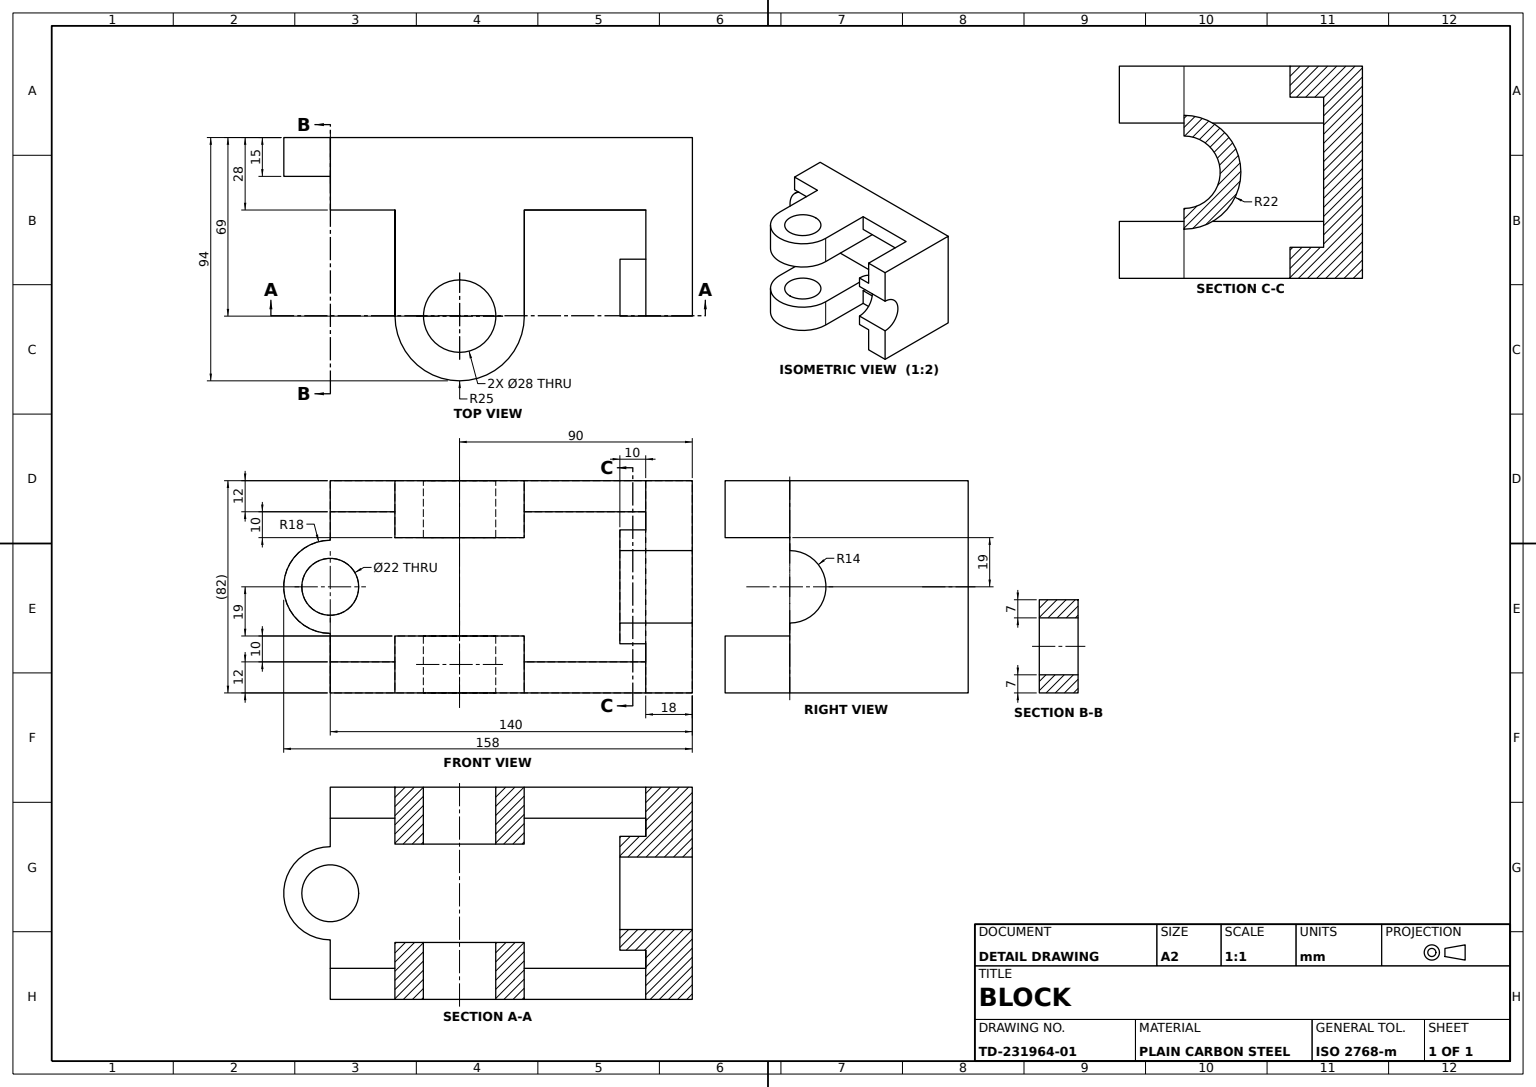
from build123d import *

# Parameters (mm, degrees)
BASE_PLATE_SKETCH_W         = 140
BASE_PLATE_SKETCH_H         = 82
BASE_PLATE_DEPTH            = 15
BACK_WALL_SKETCH_W          = 54
BACK_WALL_SKETCH_H          = 82
BACK_WALL_DEPTH             = 18
REAR_HALF_BOSS_DEPTH        = 10
REAR_HALF_ROUND_CUT_DEPTH   = 28
LOWER_LUG_DEPTH             = 22
SPACER_BLOCK_1_SKETCH_W     = 47
SPACER_BLOCK_1_SKETCH_H     = 13
SPACER_BLOCK_1_DEPTH        = 12
SPACER_BLOCK_2_SKETCH_W     = 25
SPACER_BLOCK_2_SKETCH_H     = 13
SPACER_BLOCK_2_DEPTH        = 12
SPACER_BLOCK_3_SKETCH_W     = 47
SPACER_BLOCK_3_SKETCH_H     = 13
SPACER_BLOCK_3_DEPTH        = 12
UPPER_START                 = -22
UPPER_LUG_DEPTH             = 22
SPACER_BLOCK_4_SKETCH_W     = 25
SPACER_BLOCK_4_SKETCH_H     = 13
SPACER_BLOCK_4_DEPTH        = 12
SIDE_HALF_BOSS_DEPTH        = 15
SIDE_BORE_SKETCH_R          = 11
SIDE_BORE_22_DEPTH          = 15
UPPER_PIN_HOLE_SKETCH_R     = 14
UPPER_LUG_PIN_HOLE_28_DEPTH = 22
LOWER_START                 = -22
LOWER_PIN_HOLE_SKETCH_R     = 14
LOWER_LUG_PIN_HOLE_28_DEPTH = 22


with BuildPart() as part:
    # Base Plate Sketch → Base Plate (new body)
    with BuildSketch(Plane.XY):
        with Locations((70, 41)):
            Rectangle(BASE_PLATE_SKETCH_W, BASE_PLATE_SKETCH_H)
    extrude(amount=BASE_PLATE_DEPTH)

    # Back Wall Sketch → Back Wall (add)
    with BuildSketch(Plane(origin=(140, 0, 0), x_dir=(0, 0, -1), z_dir=(1, 0, 0))):
        with Locations((-42, 41)):
            Rectangle(BACK_WALL_SKETCH_W, BACK_WALL_SKETCH_H)
    extrude(amount=-BACK_WALL_DEPTH)

    # Rear Half Boss Sketch → Rear Half Boss (add)
    with BuildSketch(Plane.ZY.offset(-122)):
        with BuildLine():
            Line((69, 63), (69, 19))
            ThreePointArc((69, 19), (47, 41), (69, 63))
        make_face()
    extrude(amount=REAR_HALF_BOSS_DEPTH)

    # Rear Half-Round Cut Sketch → Rear Half-Round Cut (cut)
    with BuildSketch(Plane.ZY.offset(-112)):
        with BuildLine():
            Line((69, 55), (69, 27))
            ThreePointArc((69, 27), (55, 41), (69, 55))
        make_face()
    extrude(amount=-REAR_HALF_ROUND_CUT_DEPTH, mode=Mode.SUBTRACT)

    # Lower Lug Sketch → Lower Lug (add)
    with BuildSketch(Plane.XZ):
        with BuildLine():
            Line((75, 69), (75, 15))
            Line((75, 15), (25, 15))
            Line((25, 15), (25, 69))
            ThreePointArc((25, 69), (50, 94), (75, 69))
        make_face()
    extrude(amount=-LOWER_LUG_DEPTH)

    # Spacer Block 1 Sketch → Spacer Block 1 (add)
    with BuildSketch(Plane.XZ):
        with Locations((98.5, 21.5)):
            Rectangle(SPACER_BLOCK_1_SKETCH_W, SPACER_BLOCK_1_SKETCH_H)
    extrude(amount=-SPACER_BLOCK_1_DEPTH)

    # Spacer Block 2 Sketch → Spacer Block 2 (add)
    with BuildSketch(Plane.XZ):
        with Locations((12.5, 21.5)):
            Rectangle(SPACER_BLOCK_2_SKETCH_W, SPACER_BLOCK_2_SKETCH_H)
    extrude(amount=-SPACER_BLOCK_2_DEPTH)

    # Spacer Block 3 Sketch → Spacer Block 3 (add)
    with BuildSketch(Plane(origin=(0, 82, 0), x_dir=(1, 0, 0), z_dir=(0, 1, 0))):
        with Locations((98.5, -21.5)):
            Rectangle(SPACER_BLOCK_3_SKETCH_W, SPACER_BLOCK_3_SKETCH_H)
    extrude(amount=-SPACER_BLOCK_3_DEPTH)

    # Upper Lug Sketch → Upper Lug (add)
    with BuildSketch(Plane(origin=(0, 82, 0), x_dir=(1, 0, 0), z_dir=(0, 1, 0)).offset(UPPER_START)):
        with BuildLine():
            Line((25, -15), (75, -15))
            Line((75, -15), (75, -69))
            ThreePointArc((75, -69), (50, -94), (25, -69))
            Line((25, -69), (25, -15))
        make_face()
    extrude(amount=UPPER_LUG_DEPTH)

    # Spacer Block 4 Sketch → Spacer Block 4 (add)
    with BuildSketch(Plane(origin=(0, 82, 0), x_dir=(1, 0, 0), z_dir=(0, 1, 0))):
        with Locations((12.5, -21.5)):
            Rectangle(SPACER_BLOCK_4_SKETCH_W, SPACER_BLOCK_4_SKETCH_H)
    extrude(amount=-SPACER_BLOCK_4_DEPTH)

    # Side Half Boss Sketch → Side Half Boss (add)
    with BuildSketch(Plane.XY.offset(15)):
        with BuildLine():
            Line((0, 59), (0, 23))
            ThreePointArc((0, 23), (-18, 41), (0, 59))
        make_face()
    extrude(amount=-SIDE_HALF_BOSS_DEPTH)

    # Side Bore Sketch → Side Bore Ø22 (cut)
    with BuildSketch(Plane.XY.offset(15)):
        with Locations((0, 41)):
            Circle(SIDE_BORE_SKETCH_R)
    extrude(amount=-SIDE_BORE_22_DEPTH, mode=Mode.SUBTRACT)

    # Upper Pin Hole Sketch → Upper Lug Pin Hole Ø28 (cut)
    with BuildSketch(Plane(origin=(0, 82, 0), x_dir=(1, 0, 0), z_dir=(0, 1, 0))):
        with Locations(Location((50, -69, 0), (0, 0, 270))):
            Circle(UPPER_PIN_HOLE_SKETCH_R)
    extrude(amount=-UPPER_LUG_PIN_HOLE_28_DEPTH, mode=Mode.SUBTRACT)

    # Lower Pin Hole Sketch → Lower Lug Pin Hole Ø28 (cut)
    with BuildSketch(Plane.XZ.offset(LOWER_START)):
        with Locations(Location((50, 69, 0), (0, 0, 90))):
            Circle(LOWER_PIN_HOLE_SKETCH_R)
    extrude(amount=LOWER_LUG_PIN_HOLE_28_DEPTH, mode=Mode.SUBTRACT)


solid = part.part
